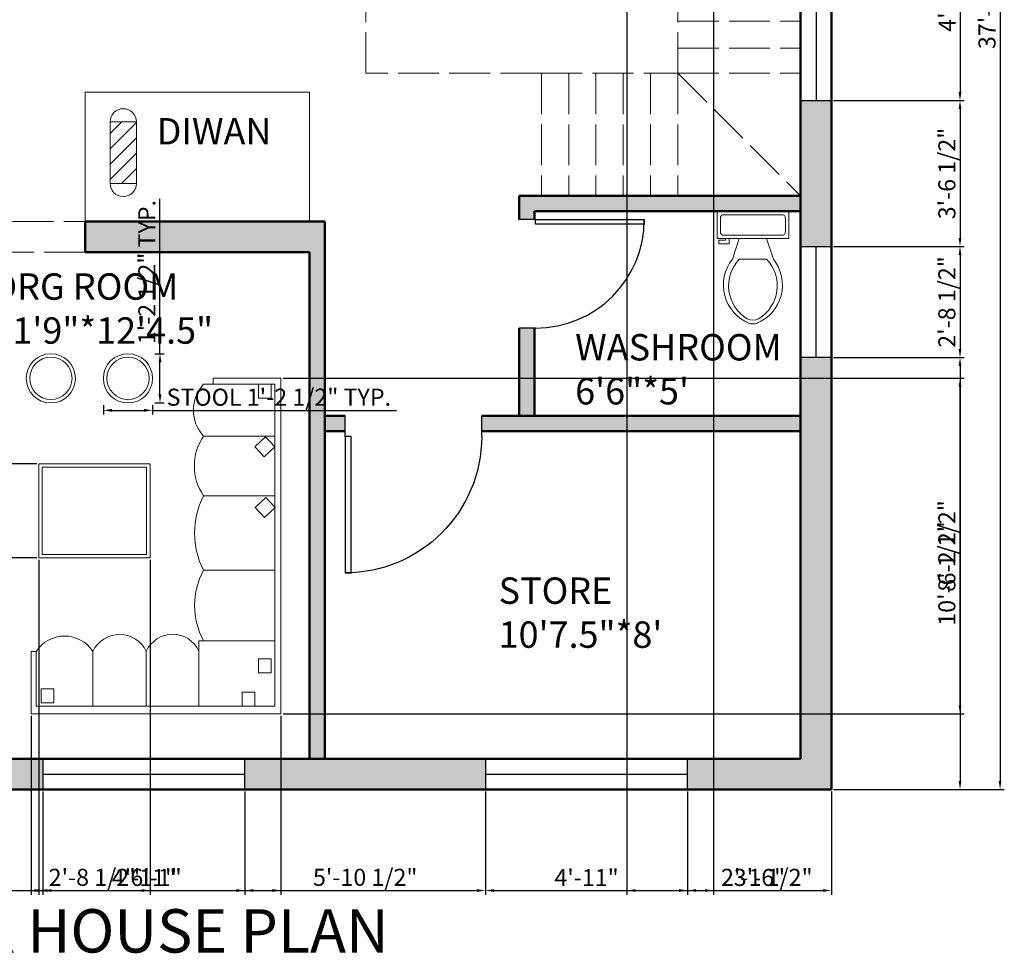
# Model space of a CAD drawing. Units: inches. Extents: x 876 to 1414, y 2665 to 3216.
# Tile 2 of 4: x 1124 to 1412, y 2665 to 2939. Entities that reach past the tile are written whole.
import ezdxf

# ---------------------------------------------------------------- set-up
doc = ezdxf.new("R2010")
doc.units = ezdxf.units.IN
doc.linetypes.add('ACAD_ISO02W100', pattern=[15, 12, -3])
for name, color, linetype, lineweight in [('A-ANNO-DIMS', 2, 'Continuous', 18), ('A-ANNO-TEXT', 7, 'Continuous', 25), ('A-AREA-IDEN', 7, 'Continuous', 25), ('A-FLOR-FIXT', 9, 'Continuous', 18), ('A-FLOR-STRS-OVHD', 150, 'ACAD_ISO02W100', 18), ('A-FURN-PATT', 252, 'Continuous', 13), ('A-OPEN-OVHD', 210, 'ACAD_ISO02W100', 18), ('A-WALL-PATT', 252, 'Continuous', 13), ('DOOR', 52, 'Continuous', 25), ('FUR', 8, 'Continuous', 18), ('WALL', 7, 'Continuous', 50), ('WIND', 130, 'Continuous', 25)]:
    doc.layers.add(name, color=color, linetype=linetype, lineweight=lineweight)
doc.styles.get("Standard").update_dxf_attribs({"font": 'arial.ttf'})
doc.dimstyles.new('ISO-25', dxfattribs={"dimtxt": 5, "dimasz": 2.5, "dimexe": 1.25, "dimexo": 0.625, "dimtad": 1, "dimdec": 0, "dimlunit": 4, "dimtxsty": 'Standard', "dimcen": 2.5, "dimadec": 0, "dimazin": 0, "dimtfac": 1, "dimtdec": 0, "dimtmove": 0, "dimatfit": 3, "dimfxl": 1, "dimarcsym": 0})

# ---------------------------------------------------------------- blocks, each defined once
blk = doc.blocks.new('*U2')
for p, q in [((0, 0), (0, -6)), ((40, 0), (40, -6))]:
    blk.add_line(p, q)
blk.add_lwpolyline([(0, 0), (0, 40), (1.75, 40), (1.75, 0)], close=True)
blk.add_arc((0, 0), 40, 0, 90)
blk = doc.blocks.new('*U6')
for p, q in [((9.5, -6), (9.5, -2)), ((-10, -8.5), (-8, -8.5)), ((-10, -9.5), (-10, -8.5)), ((-8, -8.5), (-8, -8)), ((-7, -8), (-7, -9.5)), ((-4, -8), (-6, -14)), ((4, -8), (6, -14)), ((-7, -9.5), (-10, -9.5)), ((4, -14), (-4, -14))]:
    blk.add_line(p, q)
blk.add_lwpolyline([(10.5, -8), (10.5, 0), (-10.5, 0), (-10.5, -8)], close=True)
for points in [[(-9.5, -2), (-9.5, -6)], [(8.5, -1), (-8.5, -1)], [(-8.5, -7), (8.5, -7)]]:
    blk.add_lwpolyline(points)
for centre, radius, start, end in [((-8.62, -1.88), 0.884, 81.8699, 188.1301), ((8.62, -1.88), 0.884, 351.8699, 98.1301), ((-8.62, -6.12), 0.884, 171.8699, 278.1301), ((8.62, -6.12), 0.884, 261.8699, 8.1301), ((3.52, -21.58), 12.17, 141.4691, 247.9714), ((4.2, -21.82), 11.33, 136.3677, 238.9468), ((-3.52, -21.58), 12.17, 292.0284, 38.5307), ((-4.2, -21.82), 11.33, 301.053, 43.6321), ((0, -27.88), 4, 245.7318, 294.2682), ((0, -29), 4, 254.8605, 285.1395)]:
    blk.add_arc(centre, radius, start, end)
blk = doc.blocks.new('*D8')
at = {"layer": 'A-ANNO-DIMS', "color": 0, "lineweight": -2, "transparency": 16777216}
for p, q in [((1362.14, 3166.44), (1412.22, 3166.44)), ((1410.97, 3163.94), (1410.97, 2715.94)), ((1362.14, 2713.44), (1412.22, 2713.44))]:
    blk.add_line(p, q, dxfattribs=at)
at = {"layer": 'A-ANNO-DIMS', "color": 0, "lineweight": 100, "transparency": 16777216}
for points in [[(1410.55, 3163.94), (1411.38, 3163.94), (1410.97, 3166.44)], [(1410.55, 2715.94), (1411.38, 2715.94), (1410.97, 2713.44)]]:
    blk.add_solid(points, dxfattribs=at)
at = {"layer": 'Defpoints', "color": 0, "lineweight": 100, "transparency": 16777216}
for p in [(1361.52, 3166.44), (1361.52, 2713.44), (1410.97, 2713.44)]:
    blk.add_point(p, dxfattribs=at)
at = {"layer": 'A-ANNO-DIMS', "color": 0, "transparency": 16777216, "insert": (1407.79, 2939.94), "char_height": 5, "attachment_point": 5, "rotation": 90}
blk.add_mtext('37\'-9"', dxfattribs=at)
blk = doc.blocks.new('STOOL-ROUND')
for radius in [7.21, 6.21]:
    blk.add_circle((7.21, 7.21), radius)
blk = doc.blocks.new('*D18')
at = {"layer": 'A-ANNO-DIMS', "color": 0, "lineweight": -2, "transparency": 16777216}
for p, q in [((1148.14, 2826.13), (1148.14, 2823.34)), ((1162.56, 2826.13), (1162.56, 2823.34)), ((1150.64, 2824.59), (1160.06, 2824.59)), ((1162.56, 2824.59), (1234.03, 2824.59))]:
    blk.add_line(p, q, dxfattribs=at)
at = {"layer": 'A-ANNO-DIMS', "color": 0, "lineweight": 100, "transparency": 16777216}
for points in [[(1150.64, 2825.01), (1150.64, 2824.18), (1148.14, 2824.59)], [(1160.06, 2825.01), (1160.06, 2824.18), (1162.56, 2824.59)]]:
    blk.add_solid(points, dxfattribs=at)
at = {"layer": 'Defpoints', "color": 0, "lineweight": 100, "transparency": 16777216}
for p in [(1148.14, 2826.76), (1162.56, 2826.76), (1162.56, 2824.59)]:
    blk.add_point(p, dxfattribs=at)
at = {"layer": 'A-ANNO-DIMS', "color": 0, "transparency": 16777216, "insert": (1199.55, 2827.8), "char_height": 5, "attachment_point": 5}
blk.add_mtext('STOOL 1\'-2 1/2" TYP.', dxfattribs=at)
blk = doc.blocks.new('*D19')
at = {"layer": 'A-ANNO-DIMS', "color": 0, "lineweight": -2, "transparency": 16777216}
for p, q in [((1164.72, 2841.18), (1164.72, 2886.59)), ((1163.18, 2841.18), (1165.97, 2841.18)), ((1164.72, 2829.26), (1164.72, 2838.68)), ((1163.18, 2826.76), (1165.97, 2826.76))]:
    blk.add_line(p, q, dxfattribs=at)
at = {"layer": 'A-ANNO-DIMS', "color": 0, "lineweight": 100, "transparency": 16777216}
for points in [[(1164.31, 2838.68), (1165.14, 2838.68), (1164.72, 2841.18)], [(1164.31, 2829.26), (1165.14, 2829.26), (1164.72, 2826.76)]]:
    blk.add_solid(points, dxfattribs=at)
at = {"layer": 'Defpoints', "color": 0, "lineweight": 100, "transparency": 16777216}
for p in [(1162.56, 2841.18), (1164.72, 2841.18), (1162.56, 2826.76)]:
    blk.add_point(p, dxfattribs=at)
at = {"layer": 'A-ANNO-DIMS', "color": 0, "transparency": 16777216, "insert": (1161.51, 2865.13), "char_height": 5, "attachment_point": 5, "rotation": 90}
blk.add_mtext('1\'-2 1/2" TYP.', dxfattribs=at)
blk = doc.blocks.new('*D24')
at = {"layer": 'A-ANNO-DIMS', "color": 0, "lineweight": -2, "transparency": 16777216}
for p, q in [((1301.58, 3088.78), (1301.58, 2682.56)), ((1326.96, 3088.78), (1326.96, 2682.56)), ((1304.08, 2683.81), (1324.46, 2683.81)), ((1326.96, 2683.81), (1355.74, 2683.81))]:
    blk.add_line(p, q, dxfattribs=at)
at = {"layer": 'A-ANNO-DIMS', "color": 0, "lineweight": 100, "transparency": 16777216}
for points in [[(1304.08, 2684.22), (1304.08, 2683.39), (1301.58, 2683.81)], [(1324.46, 2684.22), (1324.46, 2683.39), (1326.96, 2683.81)]]:
    blk.add_solid(points, dxfattribs=at)
at = {"layer": 'Defpoints', "color": 0, "lineweight": 100, "transparency": 16777216}
for p in [(1301.58, 3089.41), (1326.96, 3089.41), (1326.96, 2683.81)]:
    blk.add_point(p, dxfattribs=at)
at = {"layer": 'A-ANNO-DIMS', "color": 0, "transparency": 16777216, "insert": (1342.6, 2687.02), "char_height": 5, "attachment_point": 5}
blk.add_mtext('2\'-1 1/2"', dxfattribs=at)
blk = doc.blocks.new('*D28')
at = {"layer": 'A-ANNO-DIMS', "color": 0, "lineweight": -2, "transparency": 16777216}
for p, q in [((1126.95, 2735.02), (1126.95, 2682.56)), ((1200.16, 2735.02), (1200.16, 2682.56)), ((1129.45, 2683.81), (1197.66, 2683.81))]:
    blk.add_line(p, q, dxfattribs=at)
at = {"layer": 'A-ANNO-DIMS', "color": 0, "lineweight": 100, "transparency": 16777216}
for points in [[(1129.45, 2684.22), (1129.45, 2683.39), (1126.95, 2683.81)], [(1197.66, 2684.22), (1197.66, 2683.39), (1200.16, 2683.81)]]:
    blk.add_solid(points, dxfattribs=at)
at = {"layer": 'Defpoints', "color": 0, "lineweight": 100, "transparency": 16777216}
for p in [(1126.95, 2735.64), (1200.16, 2735.64), (1200.16, 2683.81)]:
    blk.add_point(p, dxfattribs=at)
at = {"layer": 'A-ANNO-DIMS', "color": 0, "transparency": 16777216, "insert": (1163.55, 2686.99), "char_height": 5, "attachment_point": 5}
blk.add_mtext('6\'-1"', dxfattribs=at)
blk = doc.blocks.new('*D29')
at = {"layer": 'A-ANNO-DIMS', "color": 0, "lineweight": -2, "transparency": 16777216}
for p, q in [((1200.79, 2834.01), (1400.48, 2834.01)), ((1399.23, 2738.14), (1399.23, 2831.51)), ((1200.79, 2735.64), (1400.48, 2735.64))]:
    blk.add_line(p, q, dxfattribs=at)
at = {"layer": 'A-ANNO-DIMS', "color": 0, "lineweight": 100, "transparency": 16777216}
for points in [[(1398.82, 2831.51), (1399.65, 2831.51), (1399.23, 2834.01)], [(1398.82, 2738.14), (1399.65, 2738.14), (1399.23, 2735.64)]]:
    blk.add_solid(points, dxfattribs=at)
at = {"layer": 'Defpoints', "color": 0, "lineweight": 100, "transparency": 16777216}
for p in [(1200.16, 2834.01), (1399.23, 2834.01), (1200.16, 2735.64)]:
    blk.add_point(p, dxfattribs=at)
at = {"layer": 'A-ANNO-DIMS', "color": 0, "transparency": 16777216, "insert": (1396.02, 2784.83), "char_height": 5, "attachment_point": 5, "rotation": 90}
blk.add_mtext('8\'-2 1/2"', dxfattribs=at)
blk = doc.blocks.new('*D30')
at = {"layer": 'A-ANNO-DIMS', "color": 0, "lineweight": -2, "transparency": 16777216}
for p, q in [((1129.2, 2780.73), (1129.2, 2682.56)), ((1161.81, 2780.73), (1161.81, 2682.56)), ((1131.7, 2683.81), (1159.31, 2683.81))]:
    blk.add_line(p, q, dxfattribs=at)
at = {"layer": 'A-ANNO-DIMS', "color": 0, "lineweight": 100, "transparency": 16777216}
for points in [[(1131.7, 2684.22), (1131.7, 2683.39), (1129.2, 2683.81)], [(1159.31, 2684.22), (1159.31, 2683.39), (1161.81, 2683.81)]]:
    blk.add_solid(points, dxfattribs=at)
at = {"layer": 'Defpoints', "color": 0, "lineweight": 100, "transparency": 16777216}
for p in [(1129.2, 2781.36), (1161.81, 2781.36), (1161.81, 2683.81)]:
    blk.add_point(p, dxfattribs=at)
at = {"layer": 'A-ANNO-DIMS', "color": 0, "transparency": 16777216, "insert": (1145.51, 2687.02), "char_height": 5, "attachment_point": 5}
blk.add_mtext('2\'-8 1/2"', dxfattribs=at)
blk = doc.blocks.new('*D31')
at = {"layer": 'A-ANNO-DIMS', "color": 0, "lineweight": -2, "transparency": 16777216}
for p, q in [((1128.58, 2808.89), (885.57, 2808.89)), ((886.82, 2783.86), (886.82, 2806.39)), ((1128.58, 2781.36), (885.57, 2781.36))]:
    blk.add_line(p, q, dxfattribs=at)
at = {"layer": 'A-ANNO-DIMS', "color": 0, "lineweight": 100, "transparency": 16777216}
for points in [[(886.4, 2806.39), (887.23, 2806.39), (886.82, 2808.89)], [(886.4, 2783.86), (887.23, 2783.86), (886.82, 2781.36)]]:
    blk.add_solid(points, dxfattribs=at)
at = {"layer": 'Defpoints', "color": 0, "lineweight": 100, "transparency": 16777216}
for p in [(886.82, 2808.89), (1129.2, 2808.89), (1129.2, 2781.36)]:
    blk.add_point(p, dxfattribs=at)
at = {"layer": 'A-ANNO-DIMS', "color": 0, "transparency": 16777216, "insert": (883.6, 2795.13), "char_height": 5, "attachment_point": 5, "rotation": 90}
blk.add_mtext('2\'-3 1/2"', dxfattribs=at)
blk = doc.blocks.new('*D42')
at = {"layer": 'A-ANNO-DIMS', "color": 0, "lineweight": -2, "transparency": 16777216}
for p, q in [((1044.28, 2710.88), (1044.28, 2682.56)), ((1130.38, 2712.82), (1130.38, 2682.56)), ((1046.78, 2683.81), (1127.88, 2683.81))]:
    blk.add_line(p, q, dxfattribs=at)
at = {"layer": 'A-ANNO-DIMS', "color": 0, "lineweight": 100, "transparency": 16777216}
for points in [[(1046.78, 2684.22), (1046.78, 2683.39), (1044.28, 2683.81)], [(1127.88, 2684.22), (1127.88, 2683.39), (1130.38, 2683.81)]]:
    blk.add_solid(points, dxfattribs=at)
at = {"layer": 'Defpoints', "color": 0, "lineweight": 100, "transparency": 16777216}
for p in [(1130.38, 2713.44), (1044.28, 2711.51), (1130.38, 2683.81)]:
    blk.add_point(p, dxfattribs=at)
at = {"layer": 'A-ANNO-DIMS', "color": 0, "transparency": 16777216, "insert": (1087.33, 2686.94), "char_height": 5, "attachment_point": 5}
blk.add_mtext('7\'-2"', dxfattribs=at)
blk = doc.blocks.new('*D43')
at = {"layer": 'A-ANNO-DIMS', "color": 0, "lineweight": -2, "transparency": 16777216}
for p, q in [((1130.38, 2712.82), (1130.38, 2682.56)), ((1189.62, 2712.82), (1189.62, 2682.56)), ((1132.88, 2683.81), (1187.12, 2683.81))]:
    blk.add_line(p, q, dxfattribs=at)
at = {"layer": 'A-ANNO-DIMS', "color": 0, "lineweight": 100, "transparency": 16777216}
for points in [[(1132.88, 2684.22), (1132.88, 2683.39), (1130.38, 2683.81)], [(1187.12, 2684.22), (1187.12, 2683.39), (1189.62, 2683.81)]]:
    blk.add_solid(points, dxfattribs=at)
at = {"layer": 'Defpoints', "color": 0, "lineweight": 100, "transparency": 16777216}
for p in [(1130.38, 2713.44), (1189.62, 2713.44), (1189.62, 2683.81)]:
    blk.add_point(p, dxfattribs=at)
at = {"layer": 'A-ANNO-DIMS', "color": 0, "transparency": 16777216, "insert": (1160, 2686.94), "char_height": 5, "attachment_point": 5}
blk.add_mtext('4\'-11"', dxfattribs=at)
blk = doc.blocks.new('*D44')
at = {"layer": 'A-ANNO-DIMS', "color": 0, "lineweight": -2, "transparency": 16777216}
for p, q in [((1189.62, 2712.82), (1189.62, 2682.56)), ((1260.12, 2712.82), (1260.12, 2682.56)), ((1192.12, 2683.81), (1257.62, 2683.81))]:
    blk.add_line(p, q, dxfattribs=at)
at = {"layer": 'A-ANNO-DIMS', "color": 0, "lineweight": 100, "transparency": 16777216}
for points in [[(1192.12, 2684.22), (1192.12, 2683.39), (1189.62, 2683.81)], [(1257.62, 2684.22), (1257.62, 2683.39), (1260.12, 2683.81)]]:
    blk.add_solid(points, dxfattribs=at)
at = {"layer": 'Defpoints', "color": 0, "lineweight": 100, "transparency": 16777216}
for p in [(1189.62, 2713.44), (1260.12, 2713.44), (1260.12, 2683.81)]:
    blk.add_point(p, dxfattribs=at)
at = {"layer": 'A-ANNO-DIMS', "color": 0, "transparency": 16777216, "insert": (1224.87, 2687.02), "char_height": 5, "attachment_point": 5}
blk.add_mtext('5\'-10 1/2"', dxfattribs=at)
blk = doc.blocks.new('*D45')
at = {"layer": 'A-ANNO-DIMS', "color": 0, "lineweight": -2, "transparency": 16777216}
for p, q in [((1260.12, 2712.82), (1260.12, 2682.56)), ((1319.37, 2712.82), (1319.37, 2682.56)), ((1262.62, 2683.81), (1316.87, 2683.81))]:
    blk.add_line(p, q, dxfattribs=at)
at = {"layer": 'A-ANNO-DIMS', "color": 0, "lineweight": 100, "transparency": 16777216}
for points in [[(1262.62, 2684.22), (1262.62, 2683.39), (1260.12, 2683.81)], [(1316.87, 2684.22), (1316.87, 2683.39), (1319.37, 2683.81)]]:
    blk.add_solid(points, dxfattribs=at)
at = {"layer": 'Defpoints', "color": 0, "lineweight": 100, "transparency": 16777216}
for p in [(1260.12, 2713.44), (1319.37, 2713.44), (1319.37, 2683.81)]:
    blk.add_point(p, dxfattribs=at)
at = {"layer": 'A-ANNO-DIMS', "color": 0, "transparency": 16777216, "insert": (1289.75, 2686.94), "char_height": 5, "attachment_point": 5}
blk.add_mtext('4\'-11"', dxfattribs=at)
blk = doc.blocks.new('*D46')
at = {"layer": 'A-ANNO-DIMS', "color": 0, "lineweight": -2, "transparency": 16777216}
for p, q in [((1319.37, 2712.82), (1319.37, 2682.56)), ((1361.52, 2712.82), (1361.52, 2682.56)), ((1321.87, 2683.81), (1359.02, 2683.81))]:
    blk.add_line(p, q, dxfattribs=at)
at = {"layer": 'A-ANNO-DIMS', "color": 0, "lineweight": 100, "transparency": 16777216}
for points in [[(1321.87, 2684.22), (1321.87, 2683.39), (1319.37, 2683.81)], [(1359.02, 2684.22), (1359.02, 2683.39), (1361.52, 2683.81)]]:
    blk.add_solid(points, dxfattribs=at)
at = {"layer": 'Defpoints', "color": 0, "lineweight": 100, "transparency": 16777216}
for p in [(1319.37, 2713.44), (1361.52, 2713.44), (1361.52, 2683.81)]:
    blk.add_point(p, dxfattribs=at)
at = {"layer": 'A-ANNO-DIMS', "color": 0, "transparency": 16777216, "insert": (1340.44, 2686.99), "char_height": 5, "attachment_point": 5}
blk.add_mtext('3\'-6"', dxfattribs=at)
blk = doc.blocks.new('*D57')
at = {"layer": 'A-ANNO-DIMS', "color": 0, "lineweight": -2, "transparency": 16777216}
for p, q in [((1362.14, 2974.65), (1400.48, 2974.65)), ((1399.23, 2972.15), (1399.23, 2917.9)), ((1362.14, 2915.4), (1400.48, 2915.4))]:
    blk.add_line(p, q, dxfattribs=at)
at = {"layer": 'A-ANNO-DIMS', "color": 0, "lineweight": 100, "transparency": 16777216}
for points in [[(1398.82, 2972.15), (1399.65, 2972.15), (1399.23, 2974.65)], [(1398.82, 2917.9), (1399.65, 2917.9), (1399.23, 2915.4)]]:
    blk.add_solid(points, dxfattribs=at)
at = {"layer": 'Defpoints', "color": 0, "lineweight": 100, "transparency": 16777216}
for p in [(1361.52, 2974.65), (1361.52, 2915.4), (1399.23, 2915.4)]:
    blk.add_point(p, dxfattribs=at)
at = {"layer": 'A-ANNO-DIMS', "color": 0, "transparency": 16777216, "insert": (1396.1, 2945.02), "char_height": 5, "attachment_point": 5, "rotation": 90}
blk.add_mtext('4\'-11"', dxfattribs=at)
blk = doc.blocks.new('*D58')
at = {"layer": 'A-ANNO-DIMS', "color": 0, "lineweight": -2, "transparency": 16777216}
for p, q in [((1362.14, 2915.4), (1400.48, 2915.4)), ((1399.23, 2912.9), (1399.23, 2875.16)), ((1362.14, 2872.66), (1400.48, 2872.66))]:
    blk.add_line(p, q, dxfattribs=at)
at = {"layer": 'A-ANNO-DIMS', "color": 0, "lineweight": 100, "transparency": 16777216}
for points in [[(1398.82, 2912.9), (1399.65, 2912.9), (1399.23, 2915.4)], [(1398.82, 2875.16), (1399.65, 2875.16), (1399.23, 2872.66)]]:
    blk.add_solid(points, dxfattribs=at)
at = {"layer": 'Defpoints', "color": 0, "lineweight": 100, "transparency": 16777216}
for p in [(1361.52, 2915.4), (1361.52, 2872.66), (1399.23, 2872.66)]:
    blk.add_point(p, dxfattribs=at)
at = {"layer": 'A-ANNO-DIMS', "color": 0, "transparency": 16777216, "insert": (1396.02, 2894.03), "char_height": 5, "attachment_point": 5, "rotation": 90}
blk.add_mtext('3\'-6 1/2"', dxfattribs=at)
blk = doc.blocks.new('*D59')
at = {"layer": 'A-ANNO-DIMS', "color": 0, "lineweight": -2, "transparency": 16777216}
for p, q in [((1362.14, 2872.66), (1400.48, 2872.66)), ((1399.23, 2870.16), (1399.23, 2842.55)), ((1362.14, 2840.05), (1400.48, 2840.05))]:
    blk.add_line(p, q, dxfattribs=at)
at = {"layer": 'A-ANNO-DIMS', "color": 0, "lineweight": 100, "transparency": 16777216}
for points in [[(1398.82, 2870.16), (1399.65, 2870.16), (1399.23, 2872.66)], [(1398.82, 2842.55), (1399.65, 2842.55), (1399.23, 2840.05)]]:
    blk.add_solid(points, dxfattribs=at)
at = {"layer": 'Defpoints', "color": 0, "lineweight": 100, "transparency": 16777216}
for p in [(1361.52, 2872.66), (1361.52, 2840.05), (1399.23, 2840.05)]:
    blk.add_point(p, dxfattribs=at)
at = {"layer": 'A-ANNO-DIMS', "color": 0, "transparency": 16777216, "insert": (1396.02, 2856.36), "char_height": 5, "attachment_point": 5, "rotation": 90}
blk.add_mtext('2\'-8 1/2"', dxfattribs=at)
blk = doc.blocks.new('*D60')
at = {"layer": 'A-ANNO-DIMS', "color": 0, "lineweight": -2, "transparency": 16777216}
for p, q in [((1362.14, 2840.05), (1400.48, 2840.05)), ((1399.23, 2837.55), (1399.23, 2715.94)), ((1362.14, 2713.44), (1400.48, 2713.44))]:
    blk.add_line(p, q, dxfattribs=at)
at = {"layer": 'A-ANNO-DIMS', "color": 0, "lineweight": 100, "transparency": 16777216}
for points in [[(1398.82, 2837.55), (1399.65, 2837.55), (1399.23, 2840.05)], [(1398.82, 2715.94), (1399.65, 2715.94), (1399.23, 2713.44)]]:
    blk.add_solid(points, dxfattribs=at)
at = {"layer": 'Defpoints', "color": 0, "lineweight": 100, "transparency": 16777216}
for p in [(1361.52, 2840.05), (1361.52, 2713.44), (1399.23, 2713.44)]:
    blk.add_point(p, dxfattribs=at)
at = {"layer": 'A-ANNO-DIMS', "color": 0, "transparency": 16777216, "insert": (1396.02, 2776.75), "char_height": 5, "attachment_point": 5, "rotation": 90}
blk.add_mtext('10\'-6 1/2"', dxfattribs=at)

msp = doc.modelspace()

# ---------------------------------------------------------------- hatches: boundary and pattern name
at = {"layer": 'A-FURN-PATT'}
h = msp.add_hatch(dxfattribs=at)
h.set_pattern_fill('ANSI31', color=256)
h.paths.add_polyline_path([(1157.8, 2909.18), (1150.1, 2909.18), (1150.1, 2891.11), (1157.8, 2891.11)])
at = {"layer": 'A-WALL-PATT'}
h = msp.add_hatch(color=256, dxfattribs=at)
h.dxf.hatch_style = 1
h.paths.add_polyline_path([(966.14, 3166.44), (914.52, 3166.44), (914.52, 3077.43), (923.52, 3077.43), (923.52, 3157.44), (966.14, 3157.44)])
h.paths.add_polyline_path([(1117.41, 3166.44), (1072.02, 3166.44), (1025.39, 3166.44), (1025.39, 3157.44), (1067.52, 3157.44), (1067.52, 3050.33), (1068, 3050.33), (1068, 3010.33), (1068, 3004.44), (1072.02, 3004.44), (1076.39, 3004.44), (1076.39, 3010.44), (1076.39, 3013.44), (1072.02, 3013.44), (1072.02, 3157.44), (1090.31, 3157.44), (1117.41, 3157.44)])
h.paths.add_polyline_path([(1257.93, 3166.44), (1225.02, 3166.44), (1176.66, 3166.44), (1176.66, 3157.44), (1216.02, 3157.44), (1216.02, 3013.44), (1116.28, 3013.44, -0.01877), (1116.39, 3010.44), (1116.39, 3004.44), (1225.02, 3004.44), (1225.02, 3014.27), (1225.02, 3110.94), (1249.02, 3110.94), (1251.21, 3110.94), (1251.21, 3115.44), (1225.02, 3115.44), (1225.02, 3157.44), (1257.93, 3157.44)])
h.paths.add_polyline_path([(1361.52, 3166.44), (1317.18, 3166.44), (1317.18, 3157.44), (1330.83, 3157.44), (1352.52, 3157.44), (1352.52, 3115.44), (1288.77, 3115.44), (1288.77, 3110.94), (1352.52, 3110.94), (1352.52, 3103.98), (1361.52, 3103.98), (1361.52, 3115.44)])
h.paths.add_polyline_path([(1028, 3010.33, -0.01947), (1028.12, 3013.44), (985.91, 3013.44), (985.91, 3004.44), (1028, 3004.44)])
h.paths.add_polyline_path([(953.71, 3013.44), (923.52, 3013.44), (923.52, 3018.18), (914.52, 3018.18), (914.52, 3004.44), (923.52, 3004.44), (953.71, 3004.44)])
h.paths.add_polyline_path([(958.09, 2944.44), (923.52, 2944.44), (923.52, 2945.19), (914.52, 2945.19), (914.52, 2939.94), (914.52, 2929.41), (923.52, 2929.41), (923.52, 2939.94), (958.09, 2939.94)])
h.paths.add_polyline_path([(1025.52, 3004.44), (1016.52, 3004.44), (1016.52, 2944.44), (987.59, 2944.44), (987.59, 2939.94), (1016.52, 2939.94), (1016.52, 2917.71, -0.025042), (1020.12, 2917.89), (1025.52, 2917.89), (1025.52, 2939.94)])
h.paths.add_polyline_path([(923.52, 2870.94), (923.52, 2879.94), (923.52, 2896.8), (914.52, 2896.8), (914.52, 2870.94), (914.52, 2713.44), (918.61, 2713.44), (918.61, 2722.81), (923.52, 2722.81)])
h.paths.add_polyline_path([(930.9, 2722.81), (918.61, 2722.81), (918.61, 2711.51), (930.9, 2711.51)])
h.paths.add_polyline_path([(1056.58, 2722.81), (1044.28, 2722.81), (1044.28, 2711.51), (1056.58, 2711.51)])
h.paths.add_polyline_path([(1130.38, 2722.44), (1076.52, 2722.44), (1067.52, 2722.44), (1056.58, 2722.44), (1056.58, 2713.44), (1076.52, 2713.44), (1130.38, 2713.44)])
h.paths.add_polyline_path([(1213.02, 2879.94), (1142.76, 2879.94), (1142.76, 2870.94), (1208.52, 2870.94), (1208.52, 2722.44), (1213.02, 2722.44)])
h.paths.add_polyline_path([(1219.02, 2822.94), (1213.02, 2822.94), (1213.02, 2818.44), (1219.02, 2818.44)])
h.paths.add_polyline_path([(1352.52, 2822.94), (1259.02, 2822.94), (1259.02, 2818.44), (1352.52, 2818.44)])
h.paths.add_polyline_path([(1274.52, 2848.67), (1270.02, 2848.67), (1270.02, 2822.94), (1274.52, 2822.94)])
h.paths.add_polyline_path([(1352.52, 2887.44), (1270.02, 2887.44), (1270.02, 2880.56), (1274.52, 2880.56), (1274.52, 2882.94), (1352.52, 2882.94)])
h.paths.add_polyline_path([(1361.52, 2915.4), (1352.52, 2915.4), (1352.52, 2872.66), (1361.52, 2872.66)])
h.paths.add_polyline_path([(1361.52, 2840.05), (1352.52, 2840.05), (1352.52, 2722.44), (1319.37, 2722.44), (1319.37, 2713.44), (1349.52, 2713.44), (1361.52, 2713.44)])
h.paths.add_polyline_path([(1260.12, 2722.44), (1225.02, 2722.44), (1213.02, 2722.44), (1208.52, 2722.44), (1189.62, 2722.44), (1189.62, 2713.44), (1213.02, 2713.44), (1260.12, 2713.44)])
h.paths.add_polyline_path([(1361.52, 3004.44), (1361.52, 3044.73), (1352.52, 3044.73), (1352.52, 3013.44), (1352.52, 2974.65), (1361.52, 2974.65)])
h.paths.add_polyline_path([(1352.52, 3013.44), (1288.77, 3013.44), (1288.77, 3004.44), (1352.52, 3004.44)])
h.paths.add_polyline_path([(1067.52, 2845.54), (1025.52, 2845.54), (1025.52, 2870.94), (1025.52, 2881.89), (1020.12, 2881.89), (1016.52, 2881.89), (1016.52, 2879.94), (923.52, 2879.94), (923.52, 2870.94), (1016.52, 2870.94), (1016.52, 2845.54), (1016.52, 2836.54), (1025.52, 2836.54), (1067.52, 2836.54)])
h.paths.add_polyline_path([(1076.52, 2728.79), (1073.09, 2728.79), (1067.52, 2728.79), (1067.52, 2722.44), (1076.52, 2722.44)])
h.paths.add_polyline_path([(1091.93, 2866.85), (1126.41, 2866.85), (1126.41, 2882.79), (1091.93, 2882.79)], flags=9)
h.paths.add_polyline_path([(1112.49, 2839.74), (1177.4, 2839.74), (1177.4, 2868.59), (1112.49, 2868.59)], flags=9)
h.paths.add_polyline_path([(1005.34, 2789.94), (1060.41, 2789.94), (1060.41, 2818.8), (1005.34, 2818.8)], flags=9)

# ---------------------------------------------------------------- linework, layer by layer
at = {"layer": 'A-FLOR-STRS-OVHD'}
for p, q in [((1225.02, 2923.44), (1225.02, 3004.44)), ((1316.52, 2923.44), (1316.52, 2944.44)), ((1316.52, 2938.74), (1352.52, 2938.74)), ((1316.52, 2930.74), (1352.52, 2930.74)), ((1276.52, 2923.44), (1225.02, 2923.44)), ((1276.52, 2923.44), (1276.52, 2887.44)), ((1276.52, 2923.44), (1316.52, 2923.44)), ((1284.52, 2923.44), (1284.52, 2887.44)), ((1292.52, 2923.44), (1292.52, 2887.44)), ((1300.52, 2923.44), (1300.52, 2887.44)), ((1308.52, 2923.44), (1308.52, 2887.44)), ((1316.52, 2923.44), (1316.52, 2887.44)), ((1316.52, 2923.44), (1352.52, 2923.44)), ((1316.52, 2923.44), (1352.52, 2887.44))]:
    msp.add_line(p, q, dxfattribs=at)
at = {"layer": 'A-OPEN-OVHD'}
msp.add_lwpolyline([(1076.52, 2879.94), (1142.76, 2879.94), (1142.76, 2870.94), (1076.52, 2870.94)], close=True, dxfattribs=at)
at = {"layer": 'FUR'}
for p, q in [((1142.76, 2879.94), (1142.76, 2917.91)), ((1142.76, 2917.91), (1208.57, 2917.91)), ((1208.57, 2917.91), (1208.57, 2879.94)), ((1180.26, 2832.24), (1180.26, 2834.01)), ((1180.26, 2834.01), (1200.16, 2834.01)), ((1200.16, 2834.01), (1200.16, 2755.18)), ((1177.49, 2817.05), (1198.34, 2817.05)), ((1177.49, 2799.56), (1198.34, 2799.56)), ((1177.49, 2777.69), (1198.34, 2777.69)), ((1176.14, 2757.03), (1176.14, 2737.82)), ((1126.95, 2735.64), (1126.95, 2753.93)), ((1126.95, 2753.93), (1128.46, 2753.93)), ((1145.04, 2753.93), (1145.04, 2737.82)), ((1160.71, 2753.93), (1160.71, 2737.82)), ((1200.16, 2755.18), (1200.16, 2735.64)), ((1200.16, 2735.64), (1126.95, 2735.64))]:
    msp.add_line(p, q, dxfattribs=at)
for points in [[(1150.1, 2891.11), (1157.8, 2891.11), (1157.8, 2909.18), (1150.1, 2909.18)], [(1193.57, 2832.24), (1197.29, 2832.24), (1197.29, 2828.14), (1193.57, 2828.14)], [(1198.37, 2813.88), (1195.24, 2810.97), (1192.54, 2813.88), (1195.67, 2816.79)], [(1129.2, 2781.36), (1161.81, 2781.36), (1161.81, 2808.89), (1129.2, 2808.89)], [(1130.2, 2782.36), (1160.81, 2782.36), (1160.81, 2807.89), (1130.2, 2807.89)], [(1198.48, 2796.11), (1195.34, 2793.2), (1192.64, 2796.11), (1195.78, 2799.02)], [(1193.57, 2751.76), (1197.29, 2751.76), (1197.29, 2747.66), (1193.57, 2747.66)], [(1129.85, 2742.93), (1133.57, 2742.93), (1133.57, 2738.83), (1129.85, 2738.83)], [(1188.83, 2741.92), (1192.56, 2741.92), (1192.56, 2737.82), (1188.83, 2737.82)]]:
    msp.add_lwpolyline(points, close=True, dxfattribs=at)
for points in [[(1177.49, 2757.03), (1198.34, 2757.03), (1198.34, 2832.24), (1177.49, 2832.24)], [(1128.46, 2753.93), (1128.46, 2737.82), (1198.34, 2737.82), (1198.34, 2757.03), (1176.14, 2757.03)]]:
    msp.add_lwpolyline(points, dxfattribs=at)
for centre, radius, start, end in [((1153.95, 2909.18), 3.85, 0, 180), ((1153.95, 2891.11), 3.85, 180, 0), ((1185.75, 2824.65), 11.22, 137.4175, 222.5825), ((1190.3, 2808.3), 15.51, 145.6622, 214.3378), ((1198.91, 2788.62), 24.05, 152.9556, 207.0444), ((1196.52, 2767.36), 21.65, 151.509, 208.491), ((1136.75, 2748.53), 9.89, 33.0652, 146.9348), ((1152.88, 2750.23), 8.66, 25.2379, 154.7621), ((1168.43, 2750.51), 8.44, 23.8926, 156.1074)]:
    msp.add_arc(centre, radius, start, end, dxfattribs=at)
at = {"layer": 'WALL'}
for p, q in [((1352.52, 3013.44), (1352.52, 2722.44)), ((1361.52, 3004.44), (1361.52, 2713.44)), ((1352.52, 2887.44), (1270.02, 2887.44)), ((1270.02, 2887.44), (1270.02, 2880.56)), ((1361.52, 2822.94), (1361.52, 2887.44)), ((1352.52, 2882.94), (1274.52, 2882.94)), ((1274.52, 2882.94), (1274.52, 2880.56)), ((1352.52, 2822.94), (1352.52, 2882.94)), ((1213.02, 2879.94), (1142.76, 2879.94)), ((1142.76, 2879.94), (1142.76, 2870.94)), ((1213.02, 2722.44), (1213.02, 2879.94)), ((1208.52, 2870.94), (1142.76, 2870.94)), ((1208.52, 2722.44), (1208.52, 2870.94)), ((1270.02, 2848.67), (1270.02, 2822.94)), ((1274.52, 2848.67), (1274.52, 2822.94)), ((1219.02, 2822.94), (1213.02, 2822.94)), ((1352.52, 2822.94), (1259.02, 2822.94)), ((1352.52, 2818.44), (1352.52, 2822.94)), ((1361.52, 2713.44), (1361.52, 2822.94)), ((1219.02, 2818.44), (1213.02, 2818.44)), ((1352.52, 2818.44), (1259.02, 2818.44)), ((1352.52, 2722.44), (1352.52, 2818.44)), ((1076.52, 2722.44), (1208.52, 2722.44)), ((1208.52, 2722.44), (1213.02, 2722.44)), ((1225.02, 2722.44), (1213.02, 2722.44)), ((1225.02, 2722.44), (1352.52, 2722.44)), ((1076.52, 2713.44), (1213.02, 2713.44)), ((1213.02, 2713.44), (1349.52, 2713.44)), ((1361.52, 2713.44), (1349.52, 2713.44))]:
    msp.add_line(p, q, dxfattribs=at)
at = {"layer": 'WIND'}
for p, q in [((1357.02, 2974.65), (1357.02, 2915.4)), ((1357.02, 2840.05), (1357.02, 2872.66)), ((1130.38, 2717.94), (1189.62, 2717.94)), ((1260.12, 2717.94), (1319.37, 2717.94))]:
    msp.add_line(p, q, dxfattribs=at)
for points in [[(1352.52, 2974.65), (1352.52, 2915.4), (1361.52, 2915.4), (1361.52, 2974.65)], [(1352.52, 2872.66), (1361.52, 2872.66), (1361.52, 2840.05), (1352.52, 2840.05)], [(1130.38, 2713.44), (1189.62, 2713.44), (1189.62, 2722.44), (1130.38, 2722.44)], [(1260.12, 2713.44), (1319.37, 2713.44), (1319.37, 2722.44), (1260.12, 2722.44)]]:
    msp.add_lwpolyline(points, close=True, dxfattribs=at)

# ---------------------------------------------------------------- block references
at = {"layer": 'A-FLOR-FIXT'}
msp.add_blockref('*U6', (1338.53, 2882.94), dxfattribs=at)
at = {"layer": 'DOOR', "xscale": 0.7970934826895729, "yscale": 0.7970934826895729, "zscale": 0.7970934826895729, "rotation": 270}
msp.add_blockref('*U2', (1274.8, 2880.56), dxfattribs=at)
at = {"layer": 'DOOR', "xscale": -1, "rotation": 180}
msp.add_blockref('*U2', (1219.02, 2816.94), dxfattribs=at)
at = {"layer": 'FUR'}
for p in [(1125.52, 2826.76), (1148.13, 2826.76)]:
    msp.add_blockref('STOOL-ROUND', p, dxfattribs=at)

# ---------------------------------------------------------------- texts
at = {"layer": 'A-ANNO-TEXT', "attachment_point": 1}
for s, width, gutter_width, insert, char_height in [('DIWAN', 254.6465, 38.66, (1163.74, 2910.29), 7.733), ('2BHK HOUSE PLAN', 418.7884, 63.58, (1077.09, 2678.33), 12.7168)]:
    msp.add_mtext_dynamic_manual_height_columns(s, width=width, gutter_width=gutter_width, heights=[0], dxfattribs=dict(at, insert=insert, char_height=char_height))
at = {"layer": 'A-AREA-IDEN', "attachment_point": 1}
for s, insert, char_height in [('DRG ROOM\\P11\'9"*12\'4.5"', (1115.59, 2864.75), 7.7325), ('WASHROOM\\P6\'6"*5\'', (1286.42, 2846.95), 7.733), ('STORE\\P10\'7.5"*8\'', (1263.98, 2775.59), 7.733)]:
    msp.add_mtext_dynamic_manual_height_columns(s, width=254.6465, gutter_width=38.66, heights=[0], dxfattribs=dict(at, insert=insert, char_height=char_height))

# ---------------------------------------------------------------- dimensions: what is measured, and where the dimension line sits
at = {"layer": 'A-ANNO-DIMS'}
dim = msp.add_linear_dim(base=(1410.97, 2713.44), p1=(1361.52, 3166.44), p2=(1361.52, 2713.44), angle=90, dimstyle='ISO-25', override={"dimclrd": 0, "dimclre": 0, "dimclrt": 0}, dxfattribs=at)
dim.commit()
dim.dimension.update_dxf_attribs({"geometry": '*D8', "text_midpoint": (1410.97, 2939.94), "dimtype": 160})
for base, p1, p2, picture, middle in [((1326.96, 2683.81), (1301.58, 3089.41), (1326.96, 3089.41), '*D24', (1342.6, 2687.02)), ((1161.81, 2683.81), (1129.2, 2781.36), (1161.81, 2781.36), '*D30', (1145.51, 2687.02)), ((1200.16, 2683.81), (1126.95, 2735.64), (1200.16, 2735.64), '*D28', (1163.55, 2686.99)), ((1130.38, 2683.81), (1044.28, 2711.51), (1130.38, 2713.44), '*D42', (1087.33, 2686.94)), ((1189.62, 2683.81), (1130.38, 2713.44), (1189.62, 2713.44), '*D43', (1160, 2686.94)), ((1260.12, 2683.81), (1189.62, 2713.44), (1260.12, 2713.44), '*D44', (1224.87, 2687.02)), ((1319.372, 2683.8073), (1260.1232, 2713.4415), (1319.372, 2713.4415), '*D45', (1289.7476, 2686.9425)), ((1361.5167, 2683.8073), (1319.372, 2713.4415), (1361.5167, 2713.4415), '*D46', (1340.4444, 2686.9868))]:
    dim = msp.add_linear_dim(base=base, p1=p1, p2=p2, dimstyle='ISO-25', override={"dimdec": 1, "dimlfac": 1, "dimrnd": 0, "dimzin": 1, "dimdsep": 46, "dimlunit": 4, "dimfrac": 2}, dxfattribs=at)
    dim.commit()
    dim.dimension.update_dxf_attribs({"geometry": picture, "text_midpoint": middle})
for base, p1, p2, picture, middle in [((1399.2325, 2915.3996), (1361.5167, 2974.6484), (1361.5167, 2915.3996), '*D57', (1396.0973, 2945.024)), ((1399.23, 2872.66), (1361.52, 2915.4), (1361.52, 2872.66), '*D58', (1396.02, 2894.03)), ((1399.23, 2840.05), (1361.52, 2872.66), (1361.52, 2840.05), '*D59', (1396.02, 2856.36)), ((1399.23, 2713.44), (1361.52, 2840.05), (1361.52, 2713.44), '*D60', (1396.02, 2776.75)), ((1399.23, 2834.01), (1200.16, 2735.64), (1200.16, 2834.01), '*D29', (1396.02, 2784.83)), ((886.82, 2808.89), (1129.2, 2781.36), (1129.2, 2808.89), '*D31', (883.6, 2795.13))]:
    dim = msp.add_linear_dim(base=base, p1=p1, p2=p2, angle=90, dimstyle='ISO-25', override={"dimdec": 1, "dimlfac": 1, "dimrnd": 0, "dimzin": 1, "dimdsep": 46, "dimlunit": 4, "dimfrac": 2}, dxfattribs=at)
    dim.commit()
    dim.dimension.update_dxf_attribs({"geometry": picture, "text_midpoint": middle})
dim = msp.add_linear_dim(base=(1164.72, 2841.18), p1=(1162.56, 2826.76), p2=(1162.56, 2841.18), angle=90, text='<> TYP.', dimstyle='ISO-25', override={"dimdec": 1, "dimlfac": 1, "dimrnd": 0, "dimzin": 1, "dimdsep": 46, "dimlunit": 4, "dimfrac": 2}, dxfattribs=at)
dim.commit()
dim.dimension.update_dxf_attribs({"geometry": '*D19', "text_midpoint": (1161.51, 2865.13)})
dim = msp.add_linear_dim(base=(1162.56, 2824.59), p1=(1148.14, 2826.76), p2=(1162.56, 2826.76), text='STOOL <> TYP.', dimstyle='ISO-25', override={"dimdec": 1, "dimlfac": 1, "dimrnd": 0, "dimzin": 1, "dimdsep": 46, "dimlunit": 4, "dimfrac": 2}, dxfattribs=at)
dim.commit()
dim.dimension.update_dxf_attribs({"geometry": '*D18', "text_midpoint": (1199.55, 2827.8)})

doc.saveas('drawing.dxf')
